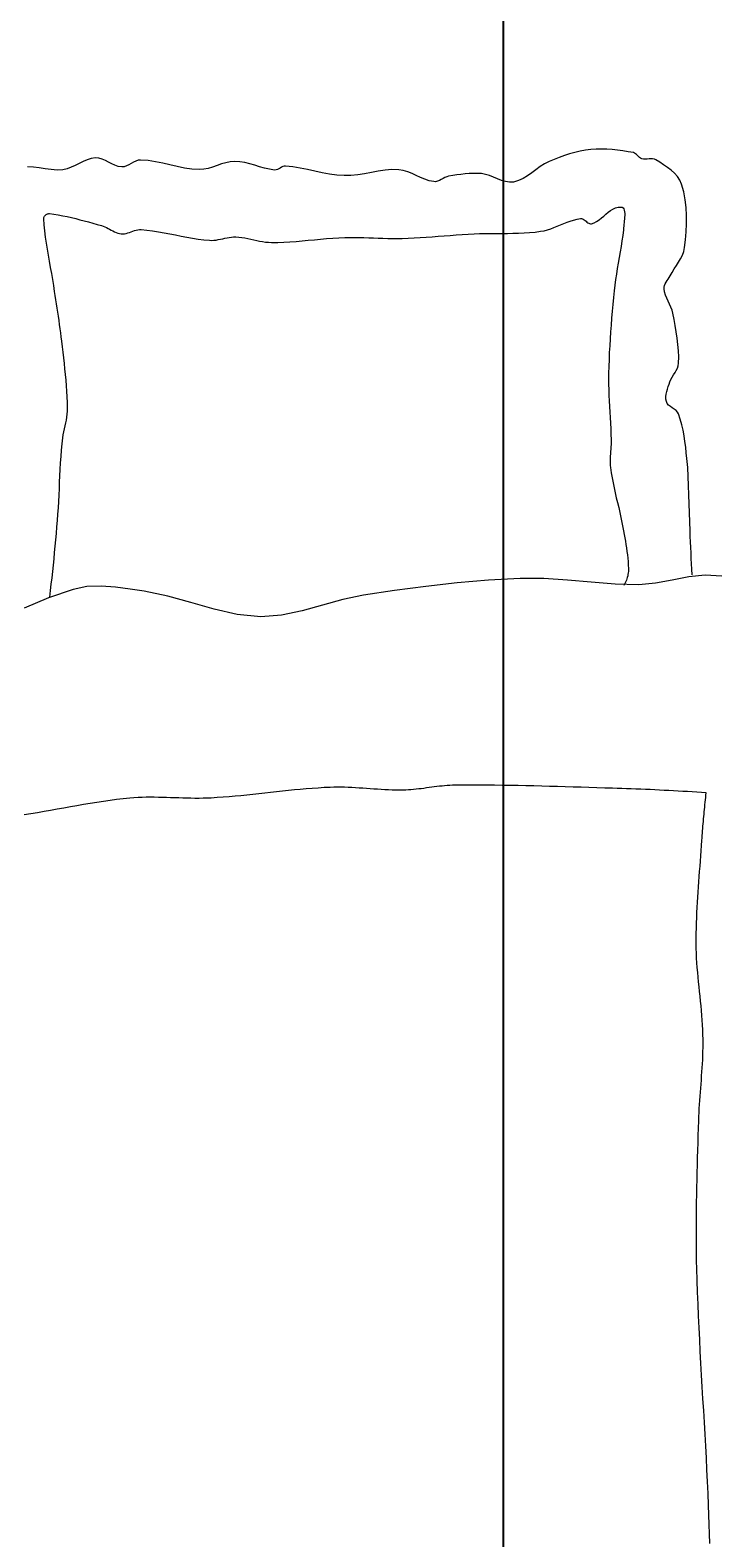
# Model space of a CAD drawing. Units: inches. Extents: x 1770 to 2988, y 1161 to 3221.
# Tile 28 of 44: x 2562 to 2593, y 2300 to 2368. Entities that reach past the tile are written whole.
import ezdxf

# ---------------------------------------------------------------- set-up
doc = ezdxf.new("R2010")
doc.units = ezdxf.units.IN
doc.layers.add('A-ANNO-DIMS', color=2, linetype='Continuous', lineweight=18)
doc.layers.add('A-FURN', color=8, linetype='Continuous', lineweight=13)
doc.styles.get("Standard").update_dxf_attribs({"font": 'arial.ttf'})
doc.dimstyles.get("Standard").update_dxf_attribs({"dimtxt": 0.18, "dimasz": 0.18, "dimexe": 0.18, "dimexo": 0.0625, "dimgap": 0.09, "dimtad": 0, "dimtih": 1, "dimtoh": 1, "dimdec": 4, "dimzin": 0, "dimdsep": 46, "dimtxsty": 'Standard', "dimcen": 0.09, "dimadec": 0, "dimazin": 0, "dimtfac": 1, "dimtdec": 4, "dimtofl": 0, "dimtmove": 0, "dimatfit": 3, "dimfxl": 1, "dimtolj": 1, "dimtzin": 0, "dimarcsym": 0})

# ---------------------------------------------------------------- blocks, each defined once
blk = doc.blocks.new('BED-DOUBLE-PLAN')
for p, q in [((61.059, 106.316), (60.819, 106.26)), ((61.3, 106.362), (61.059, 106.316)), ((61.543, 106.394), (61.3, 106.362)), ((61.783, 106.412), (61.543, 106.394)), ((62.023, 106.417), (61.783, 106.412)), ((62.265, 106.41), (62.023, 106.417)), ((62.506, 106.393), (62.265, 106.41)), ((62.747, 106.368), (62.506, 106.393)), ((62.987, 106.335), (62.747, 106.368)), ((63.226, 106.297), (62.987, 106.335)), ((63.464, 106.255), (63.226, 106.297)), ((36.348, 105.604), (36.086, 105.618)), ((38.234, 105.676), (38.054, 105.593)), ((38.413, 105.766), (38.234, 105.676)), ((38.593, 105.854), (38.413, 105.766)), ((38.774, 105.931), (38.593, 105.854)), ((38.959, 105.987), (38.774, 105.931)), ((39.151, 106.014), (38.959, 105.987)), ((39.305, 106.003), (39.151, 106.014)), ((39.454, 105.962), (39.305, 106.003)), ((39.599, 105.9), (39.454, 105.962)), ((39.744, 105.827), (39.599, 105.9)), ((39.888, 105.751), (39.744, 105.827)), ((40.034, 105.684), (39.888, 105.751)), ((40.183, 105.634), (40.034, 105.684)), ((40.337, 105.61), (40.183, 105.634)), ((40.448, 105.619), (40.337, 105.61)), ((40.556, 105.654), (40.448, 105.619)), ((40.662, 105.704), (40.556, 105.654)), ((40.766, 105.763), (40.662, 105.704)), ((40.87, 105.822), (40.766, 105.763)), ((40.976, 105.874), (40.87, 105.822)), ((41.084, 105.909), (40.976, 105.874)), ((41.195, 105.919), (41.084, 105.909)), ((41.529, 105.893), (41.195, 105.919)), ((41.861, 105.841), (41.529, 105.893)), ((42.191, 105.773), (41.861, 105.841)), ((42.521, 105.698), (42.191, 105.773)), ((42.85, 105.623), (42.521, 105.698)), ((43.18, 105.557), (42.85, 105.623)), ((44.646, 105.672), (44.449, 105.603)), ((44.844, 105.741), (44.646, 105.672)), ((45.042, 105.801), (44.844, 105.741)), ((45.243, 105.843), (45.042, 105.801)), ((45.446, 105.858), (45.243, 105.843)), ((45.675, 105.843), (45.446, 105.858)), ((45.901, 105.804), (45.675, 105.843)), ((46.126, 105.748), (45.901, 105.804)), ((46.349, 105.683), (46.126, 105.748)), ((46.572, 105.616), (46.349, 105.683)), ((46.796, 105.553), (46.572, 105.616)), ((47.615, 105.622), (47.555, 105.592)), ((47.677, 105.641), (47.615, 105.622)), ((47.741, 105.646), (47.677, 105.641)), ((48.074, 105.608), (47.741, 105.646)), ((59.252, 105.623), (59.06, 105.484)), ((59.45, 105.749), (59.252, 105.623)), ((59.658, 105.853), (59.45, 105.749)), ((59.885, 105.946), (59.658, 105.853)), ((60.115, 106.035), (59.885, 105.946)), ((60.348, 106.118), (60.115, 106.035)), ((60.582, 106.193), (60.348, 106.118)), ((60.819, 106.26), (60.582, 106.193)), ((63.519, 106.237), (63.464, 106.255)), ((63.567, 106.207), (63.519, 106.237)), ((63.612, 106.167), (63.567, 106.207)), ((63.655, 106.123), (63.612, 106.167)), ((63.698, 106.078), (63.655, 106.123)), ((63.742, 106.036), (63.698, 106.078)), ((63.79, 106), (63.742, 106.036)), ((63.842, 105.976), (63.79, 106)), ((63.921, 105.96), (63.842, 105.976)), ((64.003, 105.957), (63.921, 105.96)), ((64.087, 105.963), (64.003, 105.957)), ((64.171, 105.972), (64.087, 105.963)), ((64.255, 105.978), (64.171, 105.972)), ((64.335, 105.976), (64.255, 105.978)), ((64.412, 105.962), (64.335, 105.976)), ((64.483, 105.93), (64.412, 105.962)), ((64.655, 105.82), (64.483, 105.93)), ((64.831, 105.707), (64.655, 105.82)), ((65.005, 105.587), (64.831, 105.707)), ((36.614, 105.569), (36.348, 105.604)), ((36.882, 105.525), (36.614, 105.569)), ((37.15, 105.487), (36.882, 105.525)), ((37.417, 105.469), (37.15, 105.487)), ((37.679, 105.483), (37.417, 105.469)), ((37.869, 105.525), (37.679, 105.483)), ((38.054, 105.593), (37.869, 105.525)), ((43.512, 105.51), (43.18, 105.557)), ((43.846, 105.489), (43.512, 105.51)), ((44.05, 105.503), (43.846, 105.489)), ((44.25, 105.544), (44.05, 105.503)), ((44.449, 105.603), (44.25, 105.544)), ((47.022, 105.502), (46.796, 105.553)), ((47.25, 105.469), (47.022, 105.502)), ((47.314, 105.472), (47.25, 105.469)), ((47.375, 105.492), (47.314, 105.472)), ((47.436, 105.521), (47.375, 105.492)), ((47.495, 105.556), (47.436, 105.521)), ((47.555, 105.592), (47.495, 105.556)), ((48.406, 105.552), (48.074, 105.608)), ((48.736, 105.485), (48.406, 105.552)), ((49.065, 105.414), (48.736, 105.485)), ((49.395, 105.345), (49.065, 105.414)), ((49.725, 105.284), (49.395, 105.345)), ((50.057, 105.239), (49.725, 105.284)), ((50.391, 105.215), (50.057, 105.239)), ((50.701, 105.221), (50.391, 105.215)), ((51.01, 105.253), (50.701, 105.221)), ((51.318, 105.302), (51.01, 105.253)), ((51.626, 105.359), (51.318, 105.302)), ((51.934, 105.415), (51.626, 105.359)), ((52.242, 105.46), (51.934, 105.415)), ((52.551, 105.485), (52.242, 105.46)), ((52.86, 105.482), (52.551, 105.485)), ((53.065, 105.451), (52.86, 105.482)), ((53.264, 105.392), (53.065, 105.451)), ((53.459, 105.314), (53.264, 105.392)), ((53.652, 105.225), (53.459, 105.314)), ((53.845, 105.135), (53.652, 105.225)), ((54.039, 105.052), (53.845, 105.135)), ((54.237, 104.985), (54.039, 105.052)), ((54.441, 104.943), (54.237, 104.985)), ((54.528, 104.942), (54.441, 104.943)), ((54.613, 104.962), (54.528, 104.942)), ((54.696, 104.995), (54.613, 104.962)), ((54.779, 105.038), (54.696, 104.995)), ((54.861, 105.083), (54.779, 105.038)), ((54.944, 105.127), (54.861, 105.083)), ((55.029, 105.163), (54.944, 105.127)), ((55.116, 105.186), (55.029, 105.163)), ((55.3, 105.216), (55.116, 105.186)), ((55.484, 105.245), (55.3, 105.216)), ((55.669, 105.271), (55.484, 105.245)), ((55.855, 105.292), (55.669, 105.271)), ((56.041, 105.308), (55.855, 105.292)), ((56.227, 105.316), (56.041, 105.308)), ((56.413, 105.315), (56.227, 105.316)), ((56.598, 105.304), (56.413, 105.315)), ((56.783, 105.272), (56.598, 105.304)), ((56.966, 105.215), (56.783, 105.272)), ((57.147, 105.142), (56.966, 105.215)), ((57.327, 105.066), (57.147, 105.142)), ((57.506, 104.996), (57.327, 105.066)), ((57.686, 104.943), (57.506, 104.996)), ((57.868, 104.916), (57.686, 104.943)), ((58.051, 104.927), (57.868, 104.916)), ((58.271, 104.989), (58.051, 104.927)), ((58.479, 105.084), (58.271, 104.989)), ((58.677, 105.205), (58.479, 105.084)), ((58.869, 105.341), (58.677, 105.205)), ((59.06, 105.484), (58.869, 105.341)), ((65.17, 105.459), (65.005, 105.587)), ((65.323, 105.321), (65.17, 105.459)), ((65.456, 105.17), (65.323, 105.321)), ((65.565, 105.005), (65.456, 105.17)), ((65.644, 104.823), (65.565, 105.005)), ((65.74, 104.478), (65.644, 104.823)), ((65.806, 104.126), (65.74, 104.478)), ((62.33, 103.56), (62.435, 103.637)), ((62.435, 103.637), (62.543, 103.703)), ((62.543, 103.703), (62.655, 103.754)), ((62.655, 103.754), (62.772, 103.787)), ((62.772, 103.787), (62.895, 103.797)), ((62.895, 103.797), (62.954, 103.786)), ((62.954, 103.786), (62.999, 103.756)), ((62.999, 103.756), (63.032, 103.711)), ((63.032, 103.711), (63.054, 103.651)), ((63.054, 103.651), (63.067, 103.582)), ((63.067, 103.582), (63.073, 103.504)), ((65.847, 103.768), (65.806, 104.126)), ((65.866, 103.406), (65.847, 103.768)), ((36.815, 103.265), (36.816, 103.295)), ((36.837, 102.989), (36.815, 103.265)), ((36.816, 103.295), (36.824, 103.324)), ((36.824, 103.324), (36.836, 103.353)), ((36.836, 103.353), (36.854, 103.381)), ((36.865, 102.714), (36.837, 102.989)), ((36.854, 103.381), (36.875, 103.407)), ((36.875, 103.407), (36.9, 103.431)), ((36.9, 103.431), (36.927, 103.452)), ((36.927, 103.452), (36.956, 103.47)), ((36.956, 103.47), (36.986, 103.485)), ((36.986, 103.485), (37.017, 103.494)), ((37.017, 103.494), (37.048, 103.499)), ((37.048, 103.499), (37.077, 103.499)), ((37.077, 103.499), (37.276, 103.472)), ((37.276, 103.472), (37.474, 103.441)), ((37.474, 103.441), (37.671, 103.405)), ((37.671, 103.405), (37.868, 103.365)), ((37.868, 103.365), (38.063, 103.321)), ((38.063, 103.321), (38.259, 103.274)), ((38.259, 103.274), (38.453, 103.225)), ((38.453, 103.225), (38.648, 103.173)), ((38.648, 103.173), (38.841, 103.121)), ((38.841, 103.121), (39.035, 103.067)), ((39.035, 103.067), (39.228, 103.012)), ((39.228, 103.012), (39.421, 102.958)), ((39.421, 102.958), (39.498, 102.933)), ((39.498, 102.933), (39.573, 102.902)), ((39.573, 102.902), (39.647, 102.867)), ((59.876, 102.868), (60.024, 102.927)), ((60.024, 102.927), (60.171, 102.987)), ((60.171, 102.987), (60.319, 103.048)), ((60.319, 103.048), (60.466, 103.107)), ((60.466, 103.107), (60.615, 103.161)), ((60.615, 103.161), (60.765, 103.209)), ((60.765, 103.209), (60.917, 103.249)), ((60.917, 103.249), (61.072, 103.279)), ((61.072, 103.279), (61.117, 103.279)), ((61.117, 103.279), (61.16, 103.267)), ((61.16, 103.267), (61.202, 103.246)), ((61.202, 103.246), (61.243, 103.218)), ((61.243, 103.218), (61.284, 103.186)), ((61.284, 103.186), (61.324, 103.152)), ((61.324, 103.152), (61.364, 103.119)), ((61.364, 103.119), (61.404, 103.088)), ((61.404, 103.088), (61.445, 103.062)), ((61.445, 103.062), (61.487, 103.045)), ((61.487, 103.045), (61.529, 103.038)), ((61.529, 103.038), (61.573, 103.043)), ((61.573, 103.043), (61.691, 103.087)), ((61.691, 103.087), (61.805, 103.148)), ((61.805, 103.148), (61.914, 103.221)), ((61.914, 103.221), (62.02, 103.302)), ((62.02, 103.302), (62.123, 103.389)), ((62.123, 103.389), (62.226, 103.476)), ((62.226, 103.476), (62.33, 103.56)), ((63.038, 103.017), (63.014, 102.765)), ((63.044, 103.088), (63.038, 103.017)), ((63.053, 103.166), (63.044, 103.088)), ((63.061, 103.249), (63.053, 103.166)), ((63.069, 103.335), (63.061, 103.249)), ((63.073, 103.421), (63.069, 103.335)), ((63.073, 103.504), (63.073, 103.421)), ((65.847, 102.679), (65.864, 103.043)), ((65.864, 103.043), (65.866, 103.406)), ((36.9, 102.439), (36.865, 102.714)), ((36.939, 102.165), (36.9, 102.439)), ((39.647, 102.867), (39.721, 102.83)), ((39.721, 102.83), (39.793, 102.791)), ((39.793, 102.791), (39.866, 102.752)), ((39.866, 102.752), (39.938, 102.714)), ((39.938, 102.714), (40.011, 102.679)), ((40.011, 102.679), (40.086, 102.647)), ((40.086, 102.647), (40.161, 102.62)), ((40.161, 102.62), (40.238, 102.6)), ((40.238, 102.6), (40.317, 102.588)), ((40.317, 102.588), (40.394, 102.585)), ((40.394, 102.585), (40.469, 102.592)), ((40.469, 102.592), (40.544, 102.607)), ((40.544, 102.607), (40.619, 102.627)), ((40.619, 102.627), (40.694, 102.651)), ((40.694, 102.651), (40.769, 102.678)), ((40.769, 102.678), (40.843, 102.704)), ((40.843, 102.704), (40.918, 102.729)), ((40.918, 102.729), (40.993, 102.75)), ((40.993, 102.75), (41.068, 102.766)), ((41.068, 102.766), (41.144, 102.775)), ((41.144, 102.775), (41.22, 102.775)), ((41.22, 102.775), (41.479, 102.75)), ((41.479, 102.75), (41.737, 102.718)), ((41.737, 102.718), (41.994, 102.678)), ((41.994, 102.678), (42.251, 102.633)), ((42.251, 102.633), (42.507, 102.585)), ((42.507, 102.585), (42.763, 102.535)), ((42.763, 102.535), (43.019, 102.485)), ((43.019, 102.485), (43.275, 102.436)), ((43.275, 102.436), (43.532, 102.391)), ((43.532, 102.391), (43.789, 102.351)), ((43.789, 102.351), (44.047, 102.317)), ((44.047, 102.317), (44.306, 102.293)), ((44.306, 102.293), (44.405, 102.29)), ((44.405, 102.29), (44.505, 102.294)), ((44.505, 102.294), (44.604, 102.306)), ((44.604, 102.306), (44.703, 102.322)), ((44.703, 102.322), (44.802, 102.341)), ((44.802, 102.341), (44.902, 102.363)), ((44.902, 102.363), (45.001, 102.385)), ((45.001, 102.385), (45.1, 102.405)), ((45.1, 102.405), (45.199, 102.423)), ((45.199, 102.423), (45.299, 102.437)), ((45.299, 102.437), (45.398, 102.445)), ((45.398, 102.445), (45.498, 102.446)), ((45.498, 102.446), (45.634, 102.437)), ((45.634, 102.437), (45.769, 102.421)), ((45.769, 102.421), (45.904, 102.399)), ((45.904, 102.399), (46.038, 102.373)), ((46.038, 102.373), (46.172, 102.345)), ((46.172, 102.345), (46.306, 102.315)), ((46.306, 102.315), (46.439, 102.285)), ((46.439, 102.285), (46.573, 102.258)), ((46.573, 102.258), (46.708, 102.234)), ((46.708, 102.234), (46.842, 102.214)), ((46.842, 102.214), (46.977, 102.201)), ((47.39, 102.199), (47.666, 102.208)), ((47.666, 102.208), (47.943, 102.224)), ((47.943, 102.224), (48.219, 102.244)), ((48.219, 102.244), (48.495, 102.268)), ((48.495, 102.268), (48.771, 102.294)), ((48.771, 102.294), (49.047, 102.32)), ((49.047, 102.32), (49.323, 102.346)), ((49.323, 102.346), (49.599, 102.371)), ((49.599, 102.371), (49.876, 102.392)), ((49.876, 102.392), (50.152, 102.409)), ((50.152, 102.409), (50.429, 102.421)), ((50.429, 102.421), (50.643, 102.426)), ((50.643, 102.426), (50.858, 102.426)), ((50.858, 102.426), (51.073, 102.423)), ((51.073, 102.423), (51.288, 102.417)), ((51.288, 102.417), (51.503, 102.41)), ((51.503, 102.41), (51.718, 102.402)), ((51.718, 102.402), (51.933, 102.394)), ((51.933, 102.394), (52.148, 102.387)), ((52.148, 102.387), (52.363, 102.381)), ((52.363, 102.381), (52.578, 102.377)), ((52.578, 102.377), (52.793, 102.377)), ((52.793, 102.377), (53.008, 102.381)), ((53.008, 102.381), (53.279, 102.39)), ((53.279, 102.39), (53.551, 102.403)), ((53.551, 102.403), (53.822, 102.418)), ((53.822, 102.418), (54.093, 102.435)), ((54.093, 102.435), (54.364, 102.453)), ((54.364, 102.453), (54.635, 102.473)), ((54.635, 102.473), (54.906, 102.493)), ((54.906, 102.493), (55.177, 102.513)), ((55.177, 102.513), (55.448, 102.533)), ((55.448, 102.533), (55.719, 102.552)), ((55.719, 102.552), (55.991, 102.569)), ((55.991, 102.569), (56.262, 102.584)), ((56.262, 102.584), (56.513, 102.594)), ((56.513, 102.594), (56.764, 102.6)), ((56.764, 102.6), (57.015, 102.603)), ((57.015, 102.603), (57.267, 102.604)), ((57.267, 102.604), (57.518, 102.605)), ((57.518, 102.605), (57.77, 102.606)), ((57.77, 102.606), (58.021, 102.61)), ((58.021, 102.61), (58.272, 102.616)), ((58.272, 102.616), (58.522, 102.627)), ((58.522, 102.627), (58.773, 102.644)), ((58.773, 102.644), (59.022, 102.667)), ((59.022, 102.667), (59.271, 102.698)), ((59.271, 102.698), (59.425, 102.727)), ((59.425, 102.727), (59.578, 102.766)), ((59.578, 102.766), (59.728, 102.814)), ((59.728, 102.814), (59.876, 102.868)), ((62.949, 102.264), (62.91, 102.014)), ((62.984, 102.514), (62.949, 102.264)), ((63.014, 102.765), (62.984, 102.514)), ((65.776, 101.96), (65.816, 102.318)), ((65.816, 102.318), (65.847, 102.679)), ((36.982, 101.891), (36.939, 102.165)), ((37.028, 101.618), (36.982, 101.891)), ((37.075, 101.344), (37.028, 101.618)), ((46.977, 102.201), (47.113, 102.196)), ((47.113, 102.196), (47.39, 102.199)), ((62.869, 101.765), (62.825, 101.515)), ((62.91, 102.014), (62.869, 101.765)), ((65.6, 101.461), (65.679, 101.621)), ((65.679, 101.621), (65.74, 101.786)), ((65.74, 101.786), (65.776, 101.96)), ((37.124, 101.071), (37.075, 101.344)), ((37.173, 100.798), (37.124, 101.071)), ((62.738, 101.017), (62.697, 100.767)), ((62.781, 101.266), (62.738, 101.017)), ((62.825, 101.515), (62.781, 101.266)), ((65.126, 100.685), (65.213, 100.843)), ((65.213, 100.843), (65.309, 100.998)), ((65.309, 100.998), (65.409, 101.151)), ((65.409, 101.151), (65.508, 101.305)), ((65.508, 101.305), (65.6, 101.461)), ((37.22, 100.525), (37.173, 100.798)), ((37.265, 100.251), (37.22, 100.525)), ((37.308, 99.977), (37.265, 100.251)), ((62.624, 100.266), (62.595, 100.015)), ((62.658, 100.517), (62.624, 100.266)), ((62.697, 100.767), (62.658, 100.517)), ((64.852, 100.101), (64.855, 100.18)), ((64.855, 100.18), (64.874, 100.256)), ((64.874, 100.256), (64.906, 100.33)), ((64.906, 100.33), (64.947, 100.402)), ((64.947, 100.402), (64.993, 100.473)), ((64.993, 100.473), (65.041, 100.543)), ((65.041, 100.543), (65.086, 100.614)), ((65.086, 100.614), (65.126, 100.685)), ((37.335, 99.791), (37.308, 99.977)), ((37.364, 99.604), (37.335, 99.791)), ((37.393, 99.418), (37.364, 99.604)), ((62.564, 99.705), (62.534, 99.395)), ((62.595, 100.015), (62.564, 99.705)), ((64.874, 99.957), (64.852, 100.101)), ((64.915, 99.818), (64.874, 99.957)), ((64.97, 99.682), (64.915, 99.818)), ((65.033, 99.547), (64.97, 99.682)), ((65.098, 99.412), (65.033, 99.547)), ((37.422, 99.231), (37.393, 99.418)), ((37.451, 99.045), (37.422, 99.231)), ((37.479, 98.858), (37.451, 99.045)), ((37.507, 98.672), (37.479, 98.858)), ((62.506, 99.085), (62.479, 98.774)), ((62.534, 99.395), (62.506, 99.085)), ((65.16, 99.277), (65.098, 99.412)), ((65.212, 99.139), (65.16, 99.277)), ((65.25, 98.997), (65.212, 99.139)), ((65.304, 98.717), (65.25, 98.997)), ((37.534, 98.485), (37.507, 98.672)), ((37.56, 98.298), (37.534, 98.485)), ((37.585, 98.111), (37.56, 98.298)), ((62.432, 98.153), (62.411, 97.842)), ((62.455, 98.464), (62.432, 98.153)), ((62.479, 98.774), (62.455, 98.464)), ((65.357, 98.436), (65.304, 98.717)), ((65.405, 98.154), (65.357, 98.436)), ((65.447, 97.871), (65.405, 98.154)), ((37.609, 97.924), (37.585, 98.111)), ((37.63, 97.737), (37.609, 97.924)), ((37.659, 97.485), (37.63, 97.737)), ((37.688, 97.233), (37.659, 97.485)), ((62.393, 97.531), (62.377, 97.22)), ((62.411, 97.842), (62.393, 97.531)), ((65.481, 97.587), (65.447, 97.871)), ((65.504, 97.303), (65.481, 97.587)), ((37.717, 96.982), (37.688, 97.233)), ((37.746, 96.73), (37.717, 96.982)), ((62.364, 96.909), (62.353, 96.597)), ((62.377, 97.22), (62.364, 96.909)), ((65.515, 97.019), (65.504, 97.303)), ((65.511, 96.734), (65.515, 97.019)), ((37.774, 96.478), (37.746, 96.73)), ((37.801, 96.226), (37.774, 96.478)), ((37.825, 95.974), (37.801, 96.226)), ((62.346, 96.286), (62.343, 96.035)), ((62.353, 96.597), (62.346, 96.286)), ((65.162, 96.007), (65.218, 96.11)), ((65.218, 96.11), (65.281, 96.212)), ((65.281, 96.212), (65.346, 96.312)), ((65.346, 96.312), (65.406, 96.413)), ((65.406, 96.413), (65.458, 96.516)), ((65.458, 96.516), (65.494, 96.622)), ((65.494, 96.622), (65.511, 96.734)), ((37.846, 95.722), (37.825, 95.974)), ((37.864, 95.469), (37.846, 95.722)), ((37.877, 95.217), (37.864, 95.469)), ((62.343, 96.035), (62.346, 95.785)), ((62.346, 95.785), (62.352, 95.534)), ((62.352, 95.534), (62.362, 95.283)), ((64.948, 95.343), (64.973, 95.456)), ((64.973, 95.456), (65.006, 95.569)), ((65.006, 95.569), (65.043, 95.68)), ((65.043, 95.68), (65.082, 95.791)), ((65.082, 95.791), (65.119, 95.9)), ((65.119, 95.9), (65.162, 96.007)), ((37.886, 94.964), (37.877, 95.217)), ((37.89, 94.711), (37.886, 94.964)), ((37.886, 94.575), (37.89, 94.711)), ((62.362, 95.283), (62.374, 95.032)), ((62.374, 95.032), (62.388, 94.782)), ((62.388, 94.782), (62.403, 94.531)), ((64.935, 95.231), (64.948, 95.343)), ((64.936, 95.119), (64.935, 95.231)), ((64.955, 95.009), (64.936, 95.119)), ((64.994, 94.922), (64.955, 95.009)), ((65.057, 94.848), (64.994, 94.922)), ((65.135, 94.784), (65.057, 94.848)), ((65.222, 94.724), (65.135, 94.784)), ((65.31, 94.665), (65.222, 94.724)), ((37.783, 93.903), (37.811, 94.037)), ((37.811, 94.037), (37.836, 94.171)), ((37.836, 94.171), (37.858, 94.305)), ((37.858, 94.305), (37.875, 94.44)), ((37.875, 94.44), (37.886, 94.575)), ((62.403, 94.531), (62.417, 94.28)), ((62.417, 94.28), (62.431, 94.03)), ((62.431, 94.03), (62.443, 93.779)), ((65.391, 94.601), (65.31, 94.665)), ((65.459, 94.53), (65.391, 94.601)), ((65.505, 94.445), (65.459, 94.53)), ((65.585, 94.202), (65.505, 94.445)), ((65.653, 93.955), (65.585, 94.202)), ((37.655, 93.231), (37.676, 93.366)), ((37.676, 93.366), (37.7, 93.501)), ((37.7, 93.501), (37.727, 93.635)), ((37.727, 93.635), (37.755, 93.769)), ((37.755, 93.769), (37.783, 93.903)), ((62.443, 93.779), (62.453, 93.528)), ((62.453, 93.528), (62.46, 93.277)), ((65.709, 93.705), (65.653, 93.955)), ((65.756, 93.453), (65.709, 93.705)), ((65.796, 93.198), (65.756, 93.453)), ((37.596, 92.518), (37.616, 92.807)), ((37.616, 92.807), (37.64, 93.096)), ((37.64, 93.096), (37.655, 93.231)), ((62.435, 92.752), (62.427, 92.647)), ((62.443, 92.857), (62.435, 92.752)), ((62.451, 92.962), (62.443, 92.857)), ((62.457, 93.067), (62.451, 92.962)), ((62.46, 93.172), (62.457, 93.067)), ((62.46, 93.277), (62.46, 93.172)), ((65.829, 92.943), (65.796, 93.198)), ((65.858, 92.688), (65.829, 92.943)), ((65.884, 92.433), (65.858, 92.688)), ((37.562, 91.94), (37.578, 92.229)), ((37.578, 92.229), (37.596, 92.518)), ((62.414, 92.436), (62.411, 92.332)), ((62.411, 92.332), (62.412, 92.227)), ((62.412, 92.227), (62.418, 92.123)), ((62.419, 92.541), (62.414, 92.436)), ((62.418, 92.123), (62.429, 92.018)), ((62.427, 92.647), (62.419, 92.541)), ((62.429, 92.018), (62.462, 91.79)), ((65.919, 92.024), (65.884, 92.433)), ((65.945, 91.615), (65.919, 92.024)), ((37.521, 91.072), (37.534, 91.361)), ((37.534, 91.361), (37.548, 91.651)), ((37.548, 91.651), (37.562, 91.94)), ((62.462, 91.79), (62.502, 91.563)), ((62.502, 91.563), (62.545, 91.337)), ((62.545, 91.337), (62.593, 91.112)), ((65.963, 91.206), (65.945, 91.615)), ((37.492, 90.493), (37.507, 90.782)), ((37.507, 90.782), (37.521, 91.072)), ((62.593, 91.112), (62.643, 90.886)), ((62.643, 90.886), (62.694, 90.661)), ((62.694, 90.661), (62.747, 90.437)), ((65.977, 90.796), (65.963, 91.206)), ((65.988, 90.386), (65.977, 90.796)), ((37.457, 89.915), (37.476, 90.204)), ((37.476, 90.204), (37.492, 90.493)), ((62.747, 90.437), (62.8, 90.212)), ((62.8, 90.212), (62.851, 89.987)), ((62.851, 89.987), (62.901, 89.762)), ((65.998, 89.976), (65.988, 90.386)), ((66.01, 89.566), (65.998, 89.976)), ((37.388, 89.049), (37.412, 89.337)), ((37.412, 89.337), (37.436, 89.626)), ((37.436, 89.626), (37.457, 89.915)), ((62.901, 89.762), (62.947, 89.536)), ((62.947, 89.536), (62.99, 89.309)), ((62.99, 89.309), (63.018, 89.156)), ((66.026, 89.156), (66.01, 89.566)), ((37.336, 88.473), (37.362, 88.761)), ((37.362, 88.761), (37.388, 89.049)), ((63.018, 89.156), (63.046, 89.003)), ((63.046, 89.003), (63.074, 88.849)), ((63.074, 88.849), (63.101, 88.696)), ((63.101, 88.696), (63.128, 88.542)), ((66.037, 88.909), (66.026, 89.156)), ((66.048, 88.662), (66.037, 88.909)), ((66.059, 88.415), (66.048, 88.662)), ((37.25, 87.609), (37.279, 87.897)), ((37.279, 87.897), (37.308, 88.185)), ((37.308, 88.185), (37.336, 88.473)), ((63.128, 88.542), (63.153, 88.388)), ((63.153, 88.388), (63.175, 88.234)), ((63.175, 88.234), (63.196, 88.079)), ((63.196, 88.079), (63.213, 87.925)), ((63.213, 87.925), (63.227, 87.77)), ((66.07, 88.167), (66.059, 88.415)), ((66.081, 87.92), (66.07, 88.167)), ((66.092, 87.673), (66.081, 87.92)), ((37.188, 87.034), (37.219, 87.322)), ((37.219, 87.322), (37.25, 87.609)), ((63.23, 87.259), (63.22, 87.192)), ((63.227, 87.77), (63.236, 87.614)), ((63.237, 87.326), (63.23, 87.259)), ((63.236, 87.614), (63.241, 87.459)), ((63.241, 87.392), (63.237, 87.326)), ((63.241, 87.459), (63.241, 87.392)), ((66.104, 87.426), (66.092, 87.673)), ((66.115, 87.178), (66.104, 87.426)), ((37.121, 86.46), (37.155, 86.747)), ((37.155, 86.747), (37.188, 87.034)), ((38.769, 86.641), (38.141, 86.518)), ((39.413, 86.663), (38.769, 86.641)), ((40.065, 86.616), (39.413, 86.663)), ((40.717, 86.529), (40.065, 86.616)), ((54.088, 86.648), (52.675, 86.462)), ((55.503, 86.807), (54.088, 86.648)), ((56.922, 86.931), (55.503, 86.807)), ((58.343, 87.01), (56.922, 86.931)), ((59.417, 87.004), (58.343, 87.01)), ((60.491, 86.934), (59.417, 87.004)), ((61.564, 86.838), (60.491, 86.934)), ((62.638, 86.756), (61.564, 86.838)), ((63.713, 86.728), (62.638, 86.756)), ((63.066, 86.748), (63.033, 86.691)), ((63.097, 86.808), (63.066, 86.748)), ((63.124, 86.869), (63.097, 86.808)), ((63.149, 86.932), (63.124, 86.869)), ((63.171, 86.996), (63.149, 86.932)), ((63.19, 87.06), (63.171, 86.996)), ((63.207, 87.126), (63.19, 87.06)), ((63.22, 87.192), (63.207, 87.126)), ((64.466, 86.795), (63.713, 86.728)), ((65.218, 86.934), (64.466, 86.795)), ((65.968, 87.079), (65.218, 86.934)), ((66.715, 87.159), (65.968, 87.079)), ((67.458, 87.108), (66.715, 87.159)), ((37.023, 86.135), (35.936, 85.668)), ((38.141, 86.518), (37.023, 86.135)), ((37.087, 86.172), (37.121, 86.46)), ((41.361, 86.431), (40.717, 86.529)), ((42.419, 86.215), (41.361, 86.431)), ((43.465, 85.923), (42.419, 86.215)), ((44.51, 85.624), (43.465, 85.923)), ((50.335, 86.067), (49.413, 85.808)), ((51.266, 86.26), (50.335, 86.067)), ((52.675, 86.462), (51.266, 86.26)), ((45.561, 85.387), (44.51, 85.624)), ((46.628, 85.281), (45.561, 85.387)), ((47.567, 85.35), (46.628, 85.281)), ((48.493, 85.547), (47.567, 85.35)), ((49.413, 85.808), (48.493, 85.547)), ((40.11, 77.016), (39.811, 76.976)), ((40.411, 77.051), (40.11, 77.016)), ((40.712, 77.082), (40.411, 77.051)), ((40.894, 77.097), (40.712, 77.082)), ((41.077, 77.108), (40.894, 77.097)), ((41.261, 77.116), (41.077, 77.108)), ((41.444, 77.121), (41.261, 77.116)), ((41.627, 77.122), (41.444, 77.121)), ((41.811, 77.122), (41.627, 77.122)), ((41.995, 77.119), (41.811, 77.122)), ((42.178, 77.115), (41.995, 77.119)), ((42.362, 77.11), (42.178, 77.115)), ((42.546, 77.104), (42.362, 77.11)), ((42.73, 77.097), (42.546, 77.104)), ((42.914, 77.091), (42.73, 77.097)), ((43.097, 77.085), (42.914, 77.091)), ((43.281, 77.08), (43.097, 77.085)), ((43.465, 77.076), (43.281, 77.08)), ((43.649, 77.074), (43.465, 77.076)), ((43.833, 77.073), (43.649, 77.074)), ((44.016, 77.076), (43.833, 77.073)), ((44.2, 77.081), (44.016, 77.076)), ((44.383, 77.089), (44.2, 77.081)), ((44.652, 77.105), (44.383, 77.089)), ((44.921, 77.124), (44.652, 77.105)), ((45.19, 77.145), (44.921, 77.124)), ((45.459, 77.169), (45.19, 77.145)), ((45.727, 77.194), (45.459, 77.169)), ((45.996, 77.222), (45.727, 77.194)), ((46.264, 77.25), (45.996, 77.222)), ((46.532, 77.279), (46.264, 77.25)), ((46.8, 77.308), (46.532, 77.279)), ((47.068, 77.338), (46.8, 77.308)), ((47.337, 77.368), (47.068, 77.338)), ((47.605, 77.397), (47.337, 77.368)), ((47.873, 77.425), (47.605, 77.397)), ((48.142, 77.452), (47.873, 77.425)), ((48.41, 77.477), (48.142, 77.452)), ((48.679, 77.501), (48.41, 77.477)), ((48.948, 77.522), (48.679, 77.501)), ((49.216, 77.541), (48.948, 77.522)), ((49.486, 77.557), (49.216, 77.541)), ((49.755, 77.57), (49.486, 77.557)), ((49.92, 77.575), (49.755, 77.57)), ((50.085, 77.577), (49.92, 77.575)), ((50.25, 77.576), (50.085, 77.577)), ((50.415, 77.573), (50.25, 77.576)), ((50.581, 77.567), (50.415, 77.573)), ((50.746, 77.559), (50.581, 77.567)), ((50.911, 77.55), (50.746, 77.559)), ((51.076, 77.54), (50.911, 77.55)), ((51.241, 77.529), (51.076, 77.54)), ((51.406, 77.517), (51.241, 77.529)), ((51.571, 77.505), (51.406, 77.517)), ((51.737, 77.493), (51.571, 77.505)), ((51.902, 77.482), (51.737, 77.493)), ((52.067, 77.472), (51.902, 77.482)), ((52.232, 77.462), (52.067, 77.472)), ((52.397, 77.455), (52.232, 77.462)), ((52.562, 77.448), (52.397, 77.455)), ((52.728, 77.444), (52.562, 77.448)), ((52.893, 77.443), (52.728, 77.444)), ((53.058, 77.444), (52.893, 77.443)), ((53.176, 77.448), (53.058, 77.444)), ((53.294, 77.454), (53.176, 77.448)), ((53.411, 77.462), (53.294, 77.454)), ((53.528, 77.472), (53.411, 77.462)), ((53.646, 77.484), (53.528, 77.472)), ((53.763, 77.497), (53.646, 77.484)), ((53.88, 77.511), (53.763, 77.497)), ((53.997, 77.526), (53.88, 77.511)), ((54.114, 77.542), (53.997, 77.526)), ((54.231, 77.558), (54.114, 77.542)), ((54.348, 77.574), (54.231, 77.558)), ((54.465, 77.589), (54.348, 77.574)), ((54.582, 77.604), (54.465, 77.589)), ((54.7, 77.618), (54.582, 77.604)), ((54.817, 77.631), (54.7, 77.618)), ((54.934, 77.642), (54.817, 77.631)), ((55.051, 77.651), (54.934, 77.642)), ((55.169, 77.659), (55.051, 77.651)), ((55.286, 77.664), (55.169, 77.659)), ((55.404, 77.666), (55.286, 77.664)), ((55.76, 77.669), (55.404, 77.666)), ((56.116, 77.67), (55.76, 77.669)), ((56.472, 77.669), (56.116, 77.67)), ((56.828, 77.667), (56.472, 77.669)), ((57.184, 77.664), (56.828, 77.667)), ((57.54, 77.66), (57.184, 77.664)), ((57.896, 77.655), (57.54, 77.66)), ((58.252, 77.648), (57.896, 77.655)), ((58.608, 77.641), (58.252, 77.648)), ((58.964, 77.633), (58.608, 77.641)), ((59.32, 77.625), (58.964, 77.633)), ((59.676, 77.615), (59.32, 77.625)), ((60.032, 77.606), (59.676, 77.615)), ((60.388, 77.595), (60.032, 77.606)), ((60.744, 77.585), (60.388, 77.595)), ((61.1, 77.574), (60.744, 77.585)), ((61.456, 77.563), (61.1, 77.574)), ((61.812, 77.552), (61.456, 77.563)), ((62.168, 77.541), (61.812, 77.552)), ((62.524, 77.53), (62.168, 77.541)), ((62.736, 77.524), (62.524, 77.53)), ((62.947, 77.517), (62.736, 77.524)), ((63.159, 77.509), (62.947, 77.517)), ((63.371, 77.502), (63.159, 77.509)), ((63.583, 77.494), (63.371, 77.502)), ((63.795, 77.485), (63.583, 77.494)), ((64.006, 77.476), (63.795, 77.485)), ((64.218, 77.467), (64.006, 77.476)), ((64.43, 77.457), (64.218, 77.467)), ((64.642, 77.447), (64.43, 77.457)), ((64.853, 77.436), (64.642, 77.447)), ((65.065, 77.425), (64.853, 77.436)), ((65.276, 77.414), (65.065, 77.425)), ((65.488, 77.402), (65.276, 77.414)), ((65.7, 77.39), (65.488, 77.402)), ((65.911, 77.378), (65.7, 77.39)), ((66.123, 77.365), (65.911, 77.378)), ((66.334, 77.352), (66.123, 77.365)), ((66.546, 77.338), (66.334, 77.352)), ((66.757, 77.324), (66.546, 77.338)), ((66.71, 76.895), (66.721, 77.002)), ((66.721, 77.002), (66.733, 77.11)), ((66.733, 77.11), (66.745, 77.217)), ((66.745, 77.217), (66.757, 77.324)), ((36.23, 76.374), (35.931, 76.327)), ((36.528, 76.423), (36.23, 76.374)), ((36.827, 76.474), (36.528, 76.423)), ((37.125, 76.526), (36.827, 76.474)), ((37.423, 76.579), (37.125, 76.526)), ((37.721, 76.632), (37.423, 76.579)), ((38.019, 76.686), (37.721, 76.632)), ((38.317, 76.738), (38.019, 76.686)), ((38.615, 76.79), (38.317, 76.738)), ((38.914, 76.84), (38.615, 76.79)), ((39.212, 76.888), (38.914, 76.84)), ((39.511, 76.934), (39.212, 76.888)), ((39.811, 76.976), (39.511, 76.934)), ((66.647, 76.25), (66.657, 76.358)), ((66.657, 76.358), (66.667, 76.465)), ((66.667, 76.465), (66.677, 76.573)), ((66.677, 76.573), (66.688, 76.68)), ((66.688, 76.68), (66.699, 76.788)), ((66.699, 76.788), (66.71, 76.895)), ((66.593, 75.605), (66.601, 75.712)), ((66.601, 75.712), (66.61, 75.82)), ((66.61, 75.82), (66.619, 75.928)), ((66.619, 75.928), (66.628, 76.035)), ((66.628, 76.035), (66.637, 76.143)), ((66.637, 76.143), (66.647, 76.25)), ((66.546, 74.941), (66.562, 75.174)), ((66.562, 75.174), (66.569, 75.282)), ((66.569, 75.282), (66.577, 75.39)), ((66.577, 75.39), (66.585, 75.497)), ((66.585, 75.497), (66.593, 75.605)), ((66.495, 74.241), (66.512, 74.474)), ((66.512, 74.474), (66.53, 74.708)), ((66.53, 74.708), (66.546, 74.941)), ((66.441, 73.541), (66.459, 73.775)), ((66.459, 73.775), (66.477, 74.008)), ((66.477, 74.008), (66.495, 74.241)), ((66.391, 72.841), (66.407, 73.075)), ((66.407, 73.075), (66.424, 73.308)), ((66.424, 73.308), (66.441, 73.541)), ((66.348, 72.141), (66.361, 72.375)), ((66.361, 72.375), (66.376, 72.608)), ((66.376, 72.608), (66.391, 72.841)), ((66.318, 71.441), (66.326, 71.674)), ((66.326, 71.674), (66.337, 71.908)), ((66.337, 71.908), (66.348, 72.141)), ((66.304, 70.74), (66.307, 70.974)), ((66.307, 70.974), (66.311, 71.207)), ((66.311, 71.207), (66.318, 71.441)), ((66.304, 70.506), (66.304, 70.74)), ((66.308, 70.29), (66.304, 70.506)), ((66.315, 70.073), (66.308, 70.29)), ((66.325, 69.857), (66.315, 70.073)), ((66.338, 69.64), (66.325, 69.857)), ((66.354, 69.424), (66.338, 69.64)), ((66.372, 69.208), (66.354, 69.424)), ((66.391, 68.992), (66.372, 69.208)), ((66.412, 68.776), (66.391, 68.992)), ((66.434, 68.56), (66.412, 68.776)), ((66.456, 68.344), (66.434, 68.56)), ((66.478, 68.128), (66.456, 68.344)), ((66.5, 67.912), (66.478, 68.128)), ((66.521, 67.696), (66.5, 67.912)), ((66.541, 67.48), (66.521, 67.696)), ((66.56, 67.264), (66.541, 67.48)), ((66.577, 67.048), (66.56, 67.264)), ((66.591, 66.832), (66.577, 67.048)), ((66.603, 66.615), (66.591, 66.832)), ((66.611, 66.399), (66.603, 66.615)), ((66.616, 66.182), (66.611, 66.399)), ((66.617, 65.998), (66.616, 66.182)), ((66.597, 65.263), (66.605, 65.446)), ((66.605, 65.446), (66.611, 65.63)), ((66.611, 65.63), (66.616, 65.814)), ((66.616, 65.814), (66.617, 65.998)), ((66.563, 64.711), (66.576, 64.895)), ((66.576, 64.895), (66.587, 65.079)), ((66.587, 65.079), (66.597, 65.263)), ((66.506, 63.976), (66.521, 64.16)), ((66.521, 64.16), (66.536, 64.344)), ((66.536, 64.344), (66.55, 64.528)), ((66.55, 64.528), (66.563, 64.711)), ((66.452, 63.241), (66.465, 63.425)), ((66.465, 63.425), (66.478, 63.609)), ((66.478, 63.609), (66.492, 63.793)), ((66.492, 63.793), (66.506, 63.976)), ((66.417, 62.506), (66.423, 62.69)), ((66.423, 62.69), (66.431, 62.874)), ((66.431, 62.874), (66.441, 63.058)), ((66.441, 63.058), (66.452, 63.241)), ((66.398, 61.837), (66.407, 62.172)), ((66.407, 62.172), (66.417, 62.506)), ((66.379, 61.169), (66.389, 61.503)), ((66.389, 61.503), (66.398, 61.837)), ((66.361, 60.5), (66.37, 60.835)), ((66.37, 60.835), (66.379, 61.169)), ((66.344, 59.832), (66.352, 60.166)), ((66.352, 60.166), (66.361, 60.5)), ((66.33, 59.163), (66.337, 59.498)), ((66.337, 59.498), (66.344, 59.832)), ((66.32, 58.495), (66.324, 58.829)), ((66.324, 58.829), (66.33, 59.163)), ((66.314, 57.826), (66.316, 58.16)), ((66.316, 58.16), (66.32, 58.495)), ((66.313, 57.492), (66.314, 57.826)), ((66.313, 57.157), (66.313, 57.492)), ((66.315, 56.823), (66.313, 57.157)), ((66.319, 56.489), (66.315, 56.823)), ((66.324, 56.155), (66.319, 56.489)), ((66.332, 55.821), (66.324, 56.155)), ((66.347, 55.286), (66.332, 55.821)), ((66.365, 54.751), (66.347, 55.286)), ((66.386, 54.216), (66.365, 54.751)), ((66.409, 53.681), (66.386, 54.216)), ((66.434, 53.146), (66.409, 53.681)), ((66.461, 52.612), (66.434, 53.146)), ((66.489, 52.077), (66.461, 52.612)), ((66.518, 51.543), (66.489, 52.077)), ((66.548, 51.008), (66.518, 51.543)), ((66.579, 50.474), (66.548, 51.008)), ((66.611, 49.939), (66.579, 50.474)), ((66.642, 49.405), (66.611, 49.939)), ((66.673, 48.871), (66.642, 49.405)), ((66.704, 48.336), (66.673, 48.871)), ((66.733, 47.802), (66.704, 48.336)), ((66.762, 47.267), (66.733, 47.802)), ((66.789, 46.732), (66.762, 47.267)), ((66.815, 46.198), (66.789, 46.732)), ((66.839, 45.663), (66.815, 46.198)), ((66.86, 45.128), (66.839, 45.663)), ((66.877, 44.695), (66.86, 45.128)), ((66.894, 44.263), (66.877, 44.695)), ((66.91, 43.83), (66.894, 44.263)), ((66.927, 43.397), (66.91, 43.83))]:
    blk.add_line(p, q)
blk = doc.blocks.new('*D84')
at = {"layer": 'A-ANNO-DIMS', "color": 0, "lineweight": -2, "transparency": 16777216}
for p, q in [((2513.196, 1835.265), (2513.196, 2570.705)), ((2513.376, 2570.525), (2564.56, 2570.525)), ((2616.516, 2570.525), (2565.332, 2570.525)), ((2616.696, 1835.265), (2616.696, 2570.705))]:
    blk.add_line(p, q, dxfattribs=at)
at = {"layer": 'A-ANNO-DIMS', "color": 0, "transparency": 16777216}
for points in [[(2513.376, 2570.555), (2513.376, 2570.495), (2513.196, 2570.525)], [(2616.516, 2570.555), (2616.516, 2570.495), (2616.696, 2570.525)]]:
    blk.add_solid(points, dxfattribs=at)
at = {"layer": 'Defpoints', "color": 0, "transparency": 16777216}
for p in [(2616.696, 2570.525), (2513.196, 1835.202), (2616.696, 1835.202)]:
    blk.add_point(p, dxfattribs=at)
at = {"layer": 'A-ANNO-DIMS', "color": 0, "transparency": 16777216, "insert": (2564.946, 2570.525), "char_height": 0.18, "attachment_point": 5}
blk.add_mtext('\\A1;103.5', dxfattribs=at)
blk = doc.blocks.new('*D86')
at = {"layer": 'A-ANNO-DIMS', "color": 0, "lineweight": -2, "transparency": 16777216}
for p, q in [((2583.196, 1775.211), (2583.196, 2570.705)), ((2583.376, 2570.525), (2599.622, 2570.525)), ((2616.516, 2570.525), (2600.27, 2570.525)), ((2616.696, 1775.265), (2616.696, 2570.705))]:
    blk.add_line(p, q, dxfattribs=at)
at = {"layer": 'A-ANNO-DIMS', "color": 0, "transparency": 16777216}
for points in [[(2583.376, 2570.555), (2583.376, 2570.495), (2583.196, 2570.525)], [(2616.516, 2570.555), (2616.516, 2570.495), (2616.696, 2570.525)]]:
    blk.add_solid(points, dxfattribs=at)
at = {"layer": 'Defpoints', "color": 0, "transparency": 16777216}
for p in [(2616.696, 2570.525), (2583.196, 1775.149), (2616.696, 1775.202)]:
    blk.add_point(p, dxfattribs=at)
at = {"layer": 'A-ANNO-DIMS', "color": 0, "transparency": 16777216, "insert": (2599.946, 2570.525), "char_height": 0.18, "attachment_point": 5}
blk.add_mtext('\\A1;33.5', dxfattribs=at)

msp = doc.modelspace()

# ---------------------------------------------------------------- block references
at = {"layer": 'A-FURN'}
msp.add_blockref('BED-DOUBLE-PLAN', (2525.5949, 2255.9126), dxfattribs=at)

# ---------------------------------------------------------------- dimensions: what is measured, and where the dimension line sits
at = {"layer": 'A-ANNO-DIMS'}
for p1, p2, picture, middle in [((2513.196, 1835.2021), (2616.696, 1835.2021), '*D84', (2564.946, 2570.5247)), ((2583.196, 1775.149), (2616.696, 1775.2021), '*D86', (2599.946, 2570.5247))]:
    dim = msp.add_linear_dim(base=(2616.696, 2570.5247), p1=p1, p2=p2, dimstyle='Standard', override={"dimdec": 1, "dimlfac": 1, "dimrnd": 0, "dimzin": 0, "dimdsep": 46, "dimlunit": 2}, dxfattribs=at)
    dim.commit()
    dim.dimension.update_dxf_attribs({"geometry": picture, "text_midpoint": middle})

doc.saveas('drawing.dxf')
